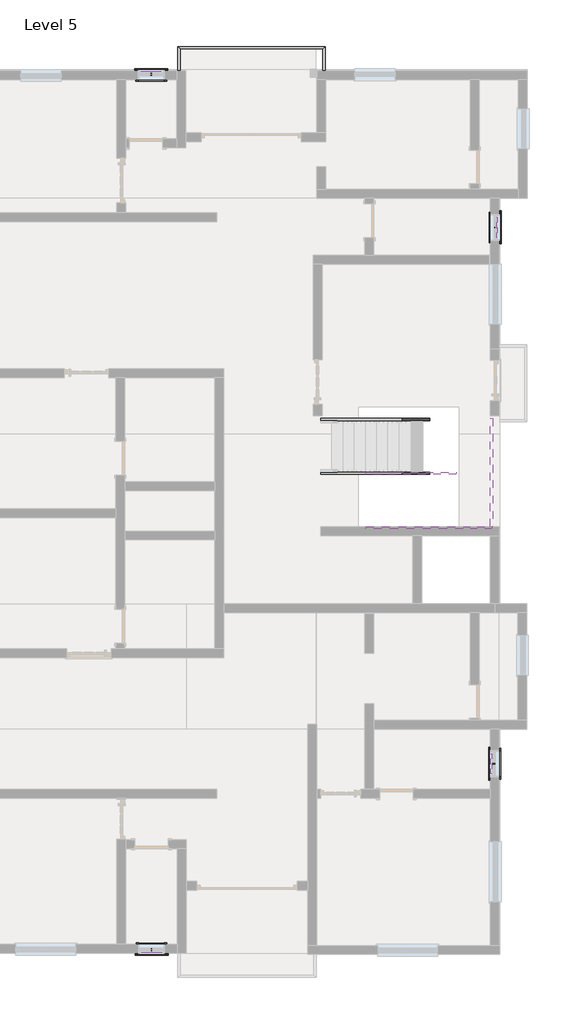
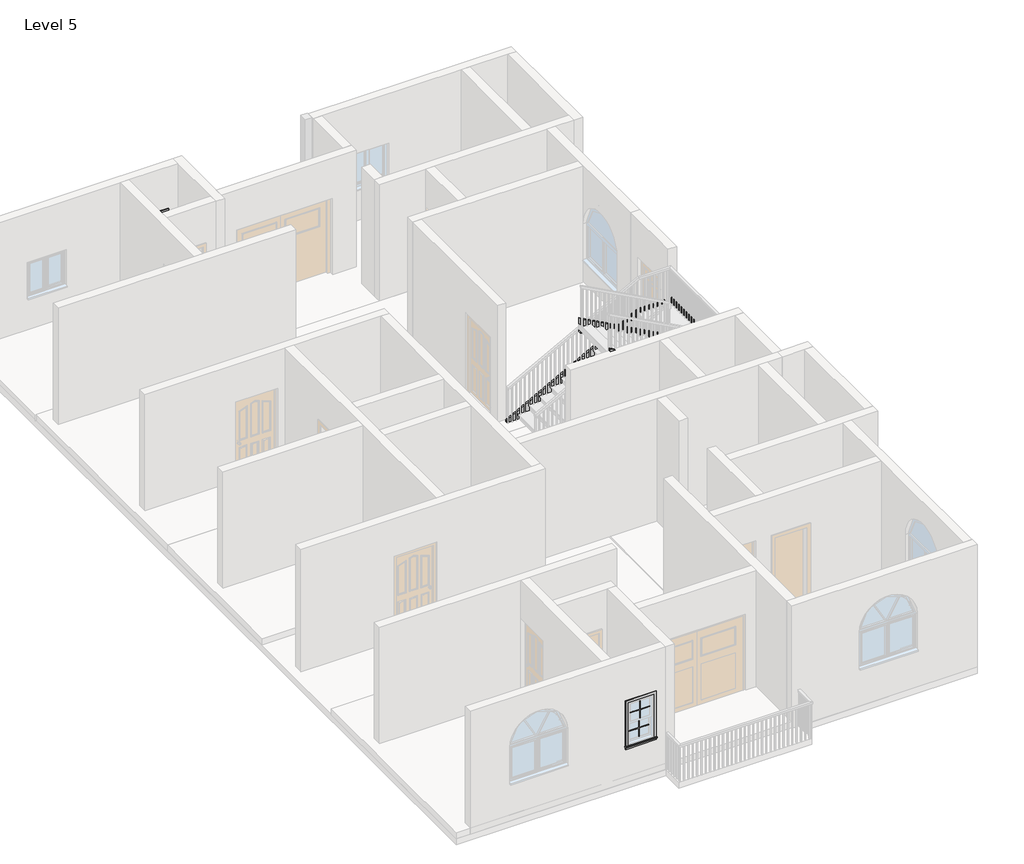
# One storey, part 7 of 7: 16 proxies, 5 members, 1 railing.
"""IFC4 building model written with IfcOpenShell, lengths in millimetres."""

from ifc_helpers import new_model, si_unit, frame, origin, place, context, project, spatial, polyline, outline, extrude, faceted_brep, transform, mapped, element, save
from components import muntin_pattern_2x2_muntin_pattern_2x2_eba6c5fb, trim_window_exterior_flat_with_sill_278e6a94, trim_window_interior_flat_picture_frame_e9fd5f45

model = new_model("IFC4")

# Units and contexts
model_context = context("Model", 3, world=origin())
ifc_project = project(units=[si_unit("LENGTHUNIT", "METRE", prefix="MILLI")], contexts=[model_context])

# Site, building, storey
site = spatial("IfcSite", under=ifc_project)
building = spatial("IfcBuilding", under=site)
storey = spatial("IfcBuildingStorey", under=building, Name="Level 5", Elevation=12192.0)

# Proxies
placement = place(None, origin())
muntin_pattern_2x2_muntin_pattern_2x2_shape = muntin_pattern_2x2_muntin_pattern_2x2_eba6c5fb(model_context)
element("IfcBuildingElementProxy", 1, Name="Muntin Pattern_2x2 : Muntin Pattern_2x2", ObjectType="Muntin Pattern_2x2 : Muntin Pattern_2x2", at=placement, inside=storey, context=model_context, shape_type="MappedRepresentation", body=[
    mapped(muntin_pattern_2x2_muntin_pattern_2x2_shape, transform((5828.2640963, 5846.2962251, 13662.025), x_axis=(0.0, -1.0, 0.0), y_axis=(1.0, 0.0, 0.0), z_axis=(0.0, 0.0, 1.0))),
])
element("IfcBuildingElementProxy", 2, Name="Muntin Pattern_2x2 : Muntin Pattern_2x2", ObjectType="Muntin Pattern_2x2 : Muntin Pattern_2x2", at=placement, inside=storey, context=model_context, shape_type="MappedRepresentation", body=[
    mapped(muntin_pattern_2x2_muntin_pattern_2x2_shape, transform((5783.8140963, 5846.2962251, 13182.6), x_axis=(0.0, -1.0, 0.0), y_axis=(1.0, 0.0, 0.0), z_axis=(0.0, 0.0, 1.0))),
])
element("IfcBuildingElementProxy", 3, Name="Muntin Pattern_2x2 : Muntin Pattern_2x2", ObjectType="Muntin Pattern_2x2 : Muntin Pattern_2x2", at=placement, inside=storey, context=model_context, shape_type="MappedRepresentation", body=[
    mapped(muntin_pattern_2x2_muntin_pattern_2x2_shape, transform((5694.9140963, -6313.9537749, 13662.025), x_axis=(0.0, 1.0, 0.0), y_axis=(-1.0, 0.0, 0.0), z_axis=(0.0, 0.0, 1.0))),
])
element("IfcBuildingElementProxy", 4, Name="Muntin Pattern_2x2 : Muntin Pattern_2x2", ObjectType="Muntin Pattern_2x2 : Muntin Pattern_2x2", at=placement, inside=storey, context=model_context, shape_type="MappedRepresentation", body=[
    mapped(muntin_pattern_2x2_muntin_pattern_2x2_shape, transform((5739.3640963, -6313.9537749, 13182.6), x_axis=(0.0, 1.0, 0.0), y_axis=(-1.0, 0.0, 0.0), z_axis=(0.0, 0.0, 1.0))),
])
element("IfcBuildingElementProxy", 5, Name="Muntin Pattern_2x2 : Muntin Pattern_2x2", ObjectType="Muntin Pattern_2x2 : Muntin Pattern_2x2", at=placement, inside=storey, context=model_context, shape_type="MappedRepresentation", body=[
    mapped(muntin_pattern_2x2_muntin_pattern_2x2_shape, transform((-2029.8609037, 9366.9277313, 13662.025), x_axis=(1.0, 0.0, 0.0), y_axis=(0.0, 1.0, 0.0), z_axis=(0.0, 0.0, 1.0))),
])
element("IfcBuildingElementProxy", 6, Name="Muntin Pattern_2x2 : Muntin Pattern_2x2", ObjectType="Muntin Pattern_2x2 : Muntin Pattern_2x2", at=placement, inside=storey, context=model_context, shape_type="MappedRepresentation", body=[
    mapped(muntin_pattern_2x2_muntin_pattern_2x2_shape, transform((-2029.8609037, 9322.4777313, 13182.6), x_axis=(1.0, 0.0, 0.0), y_axis=(0.0, 1.0, 0.0), z_axis=(0.0, 0.0, 1.0))),
])
element("IfcBuildingElementProxy", 7, Name="Muntin Pattern_2x2 : Muntin Pattern_2x2", ObjectType="Muntin Pattern_2x2 : Muntin Pattern_2x2", at=placement, inside=storey, context=model_context, shape_type="MappedRepresentation", body=[
    mapped(muntin_pattern_2x2_muntin_pattern_2x2_shape, transform((-2023.5109037, -10577.9787749, 13662.025), x_axis=(-1.0, 0.0, 0.0), y_axis=(0.0, -1.0, 0.0), z_axis=(0.0, 0.0, 1.0))),
])
element("IfcBuildingElementProxy", 8, Name="Muntin Pattern_2x2 : Muntin Pattern_2x2", ObjectType="Muntin Pattern_2x2 : Muntin Pattern_2x2", at=placement, inside=storey, context=model_context, shape_type="MappedRepresentation", body=[
    mapped(muntin_pattern_2x2_muntin_pattern_2x2_shape, transform((-2023.5109037, -10533.5287749, 13182.6), x_axis=(-1.0, 0.0, 0.0), y_axis=(0.0, -1.0, 0.0), z_axis=(0.0, 0.0, 1.0))),
])
trim_window_exterior_flat_with_sill_shape = trim_window_exterior_flat_with_sill_278e6a94(model_context)
element("IfcBuildingElementProxy", 9, Name="Trim-Window-Exterior-Flat : with Sill", ObjectType="Trim-Window-Exterior-Flat : with Sill", at=placement, inside=storey, context=model_context, shape_type="MappedRepresentation", body=[
    mapped(trim_window_exterior_flat_with_sill_shape, transform((5863.1890963, 5846.2962251, 14173.2), x_axis=(0.0, 1.0, 0.0), y_axis=(0.0, 0.0, 1.0), z_axis=(1.0, 0.0, 0.0))),
])
element("IfcBuildingElementProxy", 10, Name="Trim-Window-Exterior-Flat : with Sill", ObjectType="Trim-Window-Exterior-Flat : with Sill", at=placement, inside=storey, context=model_context, shape_type="MappedRepresentation", body=[
    mapped(trim_window_exterior_flat_with_sill_shape, transform((5659.9890963, -6313.9537749, 14173.2), x_axis=(0.0, -1.0, 0.0), y_axis=(0.0, 0.0, 1.0), z_axis=(-1.0, 0.0, 0.0))),
])
element("IfcBuildingElementProxy", 11, Name="Trim-Window-Exterior-Flat : with Sill", ObjectType="Trim-Window-Exterior-Flat : with Sill", at=placement, inside=storey, context=model_context, shape_type="MappedRepresentation", body=[
    mapped(trim_window_exterior_flat_with_sill_shape, transform((-2029.8609037, 9401.8527313, 14173.2), x_axis=(-1.0, 0.0, 0.0), y_axis=(0.0, 0.0, 1.0), z_axis=(0.0, 1.0, 0.0))),
])
element("IfcBuildingElementProxy", 12, Name="Trim-Window-Exterior-Flat : with Sill", ObjectType="Trim-Window-Exterior-Flat : with Sill", at=placement, inside=storey, context=model_context, shape_type="MappedRepresentation", body=[
    mapped(trim_window_exterior_flat_with_sill_shape, transform((-2023.5109037, -10612.9037749, 14173.2), x_axis=(1.0, 0.0, 0.0), y_axis=(0.0, 0.0, 1.0), z_axis=(0.0, -1.0, 0.0))),
])
trim_window_interior_flat_picture_frame_shape = trim_window_interior_flat_picture_frame_e9fd5f45(model_context)
element("IfcBuildingElementProxy", 13, Name="Trim-Window-Interior-Flat : Picture Frame", ObjectType="Trim-Window-Interior-Flat : Picture Frame", at=placement, inside=storey, context=model_context, shape_type="MappedRepresentation", body=[
    mapped(trim_window_interior_flat_picture_frame_shape, transform((5659.9890963, 5846.2962251, 14173.2), x_axis=(0.0, -1.0, 0.0), y_axis=(0.0, 0.0, 1.0), z_axis=(-1.0, 0.0, 0.0))),
])
element("IfcBuildingElementProxy", 14, Name="Trim-Window-Interior-Flat : Picture Frame", ObjectType="Trim-Window-Interior-Flat : Picture Frame", at=placement, inside=storey, context=model_context, shape_type="MappedRepresentation", body=[
    mapped(trim_window_interior_flat_picture_frame_shape, transform((5863.1890963, -6313.9537749, 14173.2), x_axis=(0.0, 1.0, 0.0), y_axis=(0.0, 0.0, 1.0), z_axis=(1.0, 0.0, 0.0))),
])
element("IfcBuildingElementProxy", 15, Name="Trim-Window-Interior-Flat : Picture Frame", ObjectType="Trim-Window-Interior-Flat : Picture Frame", at=placement, inside=storey, context=model_context, shape_type="MappedRepresentation", body=[
    mapped(trim_window_interior_flat_picture_frame_shape, transform((-2029.8609037, 9198.6527313, 14173.2), x_axis=(1.0, 0.0, 0.0), y_axis=(0.0, 0.0, 1.0), z_axis=(0.0, -1.0, 0.0))),
])
element("IfcBuildingElementProxy", 16, Name="Trim-Window-Interior-Flat : Picture Frame", ObjectType="Trim-Window-Interior-Flat : Picture Frame", at=placement, inside=storey, context=model_context, shape_type="MappedRepresentation", body=[
    mapped(trim_window_interior_flat_picture_frame_shape, transform((-2023.5109037, -10409.7037749, 14173.2), x_axis=(-1.0, 0.0, 0.0), y_axis=(0.0, 0.0, 1.0), z_axis=(0.0, 1.0, 0.0))),
])

# Members
element("IfcMember", 17, ObjectType="Stringer - 2\" Width", at=placement, inside=storey, context=model_context, shape_type="SweptSolid", body=[
    extrude(outline(polyline([(12399.4423129, 1811.8890963), (12192.0, 1811.8890963), (12192.0, 2068.9379367), (14069.2909091, 5536.6829612), (14069.2909091, 4896.4452154), (12399.4423129, 1811.8890963)])), frame((0.0, 1464.7962251, 0.0), z_axis=(0.0, 1.0, 0.0), x_axis=(0.0, 0.0, 1.0)), (0.0, 0.0, 1.0), 50.8),
])
element("IfcMember", 18, ObjectType="Stringer - 2\" Width", at=placement, inside=storey, context=model_context, shape_type="SweptSolid", body=[
    extrude(outline(polyline([(5659.9890963, 1515.5962251), (5710.7890963, 1515.5962251), (5710.7890963, -935.5037749), (5659.9890963, -935.5037749), (5659.9890963, 1515.5962251)])), frame((0.0, 0.0, 13764.4909091), z_axis=(0.0, 0.0, 1.0), x_axis=(1.0, 0.0, 0.0)), (0.0, 0.0, 1.0), 304.8),
])
element("IfcMember", 19, ObjectType="Stringer - 2\" Width", at=placement, inside=storey, context=model_context, shape_type="SweptSolid", body=[
    extrude(outline(polyline([(13764.4909091, 5687.6636359), (15306.0362324, 2827.8890963), (14959.7736638, 2827.8890963), (13764.4909091, 5045.2998579), (13764.4909091, 5687.6636359)])), frame((0.0, -986.3037749, 0.0), z_axis=(0.0, 1.0, 0.0), x_axis=(0.0, 0.0, 1.0)), (0.0, 0.0, 1.0), 50.8),
])
element("IfcMember", 20, ObjectType="Stringer - 2\" Width", at=placement, inside=storey, context=model_context, shape_type="SweptSolid", body=[
    extrude(outline(polyline([(12399.4423129, 1811.8890963), (12192.0, 1811.8890963), (12192.0, 2068.9379367), (13686.8485088, 4830.2326586), (14033.4462232, 4830.2326586), (12399.4423129, 1811.8890963)])), frame((0.0, 245.5962251, 0.0), z_axis=(0.0, 1.0, 0.0), x_axis=(0.0, 0.0, 1.0)), (0.0, 0.0, 1.0), 50.8),
])
element("IfcMember", 21, ObjectType="Stringer - 2\" Width", at=placement, inside=storey, context=model_context, shape_type="SweptSolid", body=[
    extrude(outline(polyline([(13853.0382157, 4881.0326586), (14199.3007843, 4881.0326586), (15306.0362324, 2827.8890963), (14959.7736638, 2827.8890963), (13853.0382157, 4881.0326586)])), frame((0.0, 245.5962251, 0.0), z_axis=(0.0, 1.0, 0.0), x_axis=(0.0, 0.0, 1.0)), (0.0, 0.0, 1.0), 50.8),
])

# Railing
element("IfcRailing", 22, ObjectType="Handrail - Rectangular", at=placement, inside=storey, context=model_context, shape_type="SolidModel", body=[
    faceted_brep([(-1426.6109037, 9402.2962251, 13106.4), (-1426.6109037, 9402.2962251, 13055.6), (-1375.8109037, 9402.2962251, 13055.6), (-1375.8109037, 9402.2962251, 13106.4), (-1426.6109037, 9948.3962251, 13106.4), (-1426.6109037, 9948.3962251, 13055.6), (-1375.8109037, 9897.5962251, 13055.6), (-1375.8109037, 9897.5962251, 13106.4), (1913.4890963, 9948.3962251, 13106.4), (1913.4890963, 9948.3962251, 13055.6), (1862.6890963, 9897.5962251, 13055.6), (1862.6890963, 9897.5962251, 13106.4), (1913.4890963, 9402.2962251, 13106.4), (1862.6890963, 9402.2962251, 13106.4), (1862.6890963, 9402.2962251, 13055.6), (1913.4890963, 9402.2962251, 13055.6)], [[[0, 1, 2, 3]], [[1, 0, 4, 5]], [[2, 1, 5, 6]], [[3, 2, 6, 7]], [[0, 3, 7, 4]], [[5, 4, 8, 9]], [[6, 5, 9, 10]], [[7, 6, 10, 11]], [[4, 7, 11, 8]], [[12, 13, 14, 15]], [[9, 8, 12, 15]], [[10, 9, 15, 14]], [[11, 10, 14, 13]], [[8, 11, 13, 12]]]),
    extrude(outline(polyline([(1878.5640963, 9424.5212251), (1897.6140963, 9424.5212251), (1897.6140963, 9405.4712251), (1878.5640963, 9405.4712251), (1878.5640963, 9424.5212251)])), frame((0.0, 0.0, 12192.0), z_axis=(0.0, 0.0, 1.0), x_axis=(1.0, 0.0, 0.0)), (0.0, 0.0, 1.0), 863.6),
    extrude(outline(polyline([(1878.5640963, 9526.1212251), (1897.6140963, 9526.1212251), (1897.6140963, 9507.0712251), (1878.5640963, 9507.0712251), (1878.5640963, 9526.1212251)])), frame((0.0, 0.0, 12192.0), z_axis=(0.0, 0.0, 1.0), x_axis=(1.0, 0.0, 0.0)), (0.0, 0.0, 1.0), 863.6),
    extrude(outline(polyline([(1878.5640963, 9627.7212251), (1897.6140963, 9627.7212251), (1897.6140963, 9608.6712251), (1878.5640963, 9608.6712251), (1878.5640963, 9627.7212251)])), frame((0.0, 0.0, 12192.0), z_axis=(0.0, 0.0, 1.0), x_axis=(1.0, 0.0, 0.0)), (0.0, 0.0, 1.0), 863.6),
    extrude(outline(polyline([(1878.5640963, 9729.3212251), (1897.6140963, 9729.3212251), (1897.6140963, 9710.2712251), (1878.5640963, 9710.2712251), (1878.5640963, 9729.3212251)])), frame((0.0, 0.0, 12192.0), z_axis=(0.0, 0.0, 1.0), x_axis=(1.0, 0.0, 0.0)), (0.0, 0.0, 1.0), 863.6),
    extrude(outline(polyline([(1878.5640963, 9830.9212251), (1897.6140963, 9830.9212251), (1897.6140963, 9811.8712251), (1878.5640963, 9811.8712251), (1878.5640963, 9830.9212251)])), frame((0.0, 0.0, 12192.0), z_axis=(0.0, 0.0, 1.0), x_axis=(1.0, 0.0, 0.0)), (0.0, 0.0, 1.0), 863.6),
    extrude(outline(polyline([(1840.4640963, 9913.4712251), (1840.4640963, 9932.5212251), (1859.5140963, 9932.5212251), (1859.5140963, 9913.4712251), (1840.4640963, 9913.4712251)])), frame((0.0, 0.0, 12192.0), z_axis=(0.0, 0.0, 1.0), x_axis=(1.0, 0.0, 0.0)), (0.0, 0.0, 1.0), 863.6),
    extrude(outline(polyline([(1738.8640963, 9913.4712251), (1738.8640963, 9932.5212251), (1757.9140963, 9932.5212251), (1757.9140963, 9913.4712251), (1738.8640963, 9913.4712251)])), frame((0.0, 0.0, 12192.0), z_axis=(0.0, 0.0, 1.0), x_axis=(1.0, 0.0, 0.0)), (0.0, 0.0, 1.0), 863.6),
    extrude(outline(polyline([(1637.2640963, 9913.4712251), (1637.2640963, 9932.5212251), (1656.3140963, 9932.5212251), (1656.3140963, 9913.4712251), (1637.2640963, 9913.4712251)])), frame((0.0, 0.0, 12192.0), z_axis=(0.0, 0.0, 1.0), x_axis=(1.0, 0.0, 0.0)), (0.0, 0.0, 1.0), 863.6),
    extrude(outline(polyline([(1535.6640963, 9913.4712251), (1535.6640963, 9932.5212251), (1554.7140963, 9932.5212251), (1554.7140963, 9913.4712251), (1535.6640963, 9913.4712251)])), frame((0.0, 0.0, 12192.0), z_axis=(0.0, 0.0, 1.0), x_axis=(1.0, 0.0, 0.0)), (0.0, 0.0, 1.0), 863.6),
    extrude(outline(polyline([(1434.0640963, 9913.4712251), (1434.0640963, 9932.5212251), (1453.1140963, 9932.5212251), (1453.1140963, 9913.4712251), (1434.0640963, 9913.4712251)])), frame((0.0, 0.0, 12192.0), z_axis=(0.0, 0.0, 1.0), x_axis=(1.0, 0.0, 0.0)), (0.0, 0.0, 1.0), 863.6),
    extrude(outline(polyline([(1332.4640963, 9913.4712251), (1332.4640963, 9932.5212251), (1351.5140963, 9932.5212251), (1351.5140963, 9913.4712251), (1332.4640963, 9913.4712251)])), frame((0.0, 0.0, 12192.0), z_axis=(0.0, 0.0, 1.0), x_axis=(1.0, 0.0, 0.0)), (0.0, 0.0, 1.0), 863.6),
    extrude(outline(polyline([(1230.8640963, 9913.4712251), (1230.8640963, 9932.5212251), (1249.9140963, 9932.5212251), (1249.9140963, 9913.4712251), (1230.8640963, 9913.4712251)])), frame((0.0, 0.0, 12192.0), z_axis=(0.0, 0.0, 1.0), x_axis=(1.0, 0.0, 0.0)), (0.0, 0.0, 1.0), 863.6),
    extrude(outline(polyline([(1129.2640963, 9913.4712251), (1129.2640963, 9932.5212251), (1148.3140963, 9932.5212251), (1148.3140963, 9913.4712251), (1129.2640963, 9913.4712251)])), frame((0.0, 0.0, 12192.0), z_axis=(0.0, 0.0, 1.0), x_axis=(1.0, 0.0, 0.0)), (0.0, 0.0, 1.0), 863.6),
    extrude(outline(polyline([(1027.6640963, 9913.4712251), (1027.6640963, 9932.5212251), (1046.7140963, 9932.5212251), (1046.7140963, 9913.4712251), (1027.6640963, 9913.4712251)])), frame((0.0, 0.0, 12192.0), z_axis=(0.0, 0.0, 1.0), x_axis=(1.0, 0.0, 0.0)), (0.0, 0.0, 1.0), 863.6),
    extrude(outline(polyline([(926.0640963, 9913.4712251), (926.0640963, 9932.5212251), (945.1140963, 9932.5212251), (945.1140963, 9913.4712251), (926.0640963, 9913.4712251)])), frame((0.0, 0.0, 12192.0), z_axis=(0.0, 0.0, 1.0), x_axis=(1.0, 0.0, 0.0)), (0.0, 0.0, 1.0), 863.6),
    extrude(outline(polyline([(824.4640963, 9913.4712251), (824.4640963, 9932.5212251), (843.5140963, 9932.5212251), (843.5140963, 9913.4712251), (824.4640963, 9913.4712251)])), frame((0.0, 0.0, 12192.0), z_axis=(0.0, 0.0, 1.0), x_axis=(1.0, 0.0, 0.0)), (0.0, 0.0, 1.0), 863.6),
    extrude(outline(polyline([(722.8640963, 9913.4712251), (722.8640963, 9932.5212251), (741.9140963, 9932.5212251), (741.9140963, 9913.4712251), (722.8640963, 9913.4712251)])), frame((0.0, 0.0, 12192.0), z_axis=(0.0, 0.0, 1.0), x_axis=(1.0, 0.0, 0.0)), (0.0, 0.0, 1.0), 863.6),
    extrude(outline(polyline([(621.2640963, 9913.4712251), (621.2640963, 9932.5212251), (640.3140963, 9932.5212251), (640.3140963, 9913.4712251), (621.2640963, 9913.4712251)])), frame((0.0, 0.0, 12192.0), z_axis=(0.0, 0.0, 1.0), x_axis=(1.0, 0.0, 0.0)), (0.0, 0.0, 1.0), 863.6),
    extrude(outline(polyline([(519.6640963, 9913.4712251), (519.6640963, 9932.5212251), (538.7140963, 9932.5212251), (538.7140963, 9913.4712251), (519.6640963, 9913.4712251)])), frame((0.0, 0.0, 12192.0), z_axis=(0.0, 0.0, 1.0), x_axis=(1.0, 0.0, 0.0)), (0.0, 0.0, 1.0), 863.6),
    extrude(outline(polyline([(418.0640963, 9913.4712251), (418.0640963, 9932.5212251), (437.1140963, 9932.5212251), (437.1140963, 9913.4712251), (418.0640963, 9913.4712251)])), frame((0.0, 0.0, 12192.0), z_axis=(0.0, 0.0, 1.0), x_axis=(1.0, 0.0, 0.0)), (0.0, 0.0, 1.0), 863.6),
    extrude(outline(polyline([(316.4640963, 9913.4712251), (316.4640963, 9932.5212251), (335.5140963, 9932.5212251), (335.5140963, 9913.4712251), (316.4640963, 9913.4712251)])), frame((0.0, 0.0, 12192.0), z_axis=(0.0, 0.0, 1.0), x_axis=(1.0, 0.0, 0.0)), (0.0, 0.0, 1.0), 863.6),
    extrude(outline(polyline([(214.8640963, 9913.4712251), (214.8640963, 9932.5212251), (233.9140963, 9932.5212251), (233.9140963, 9913.4712251), (214.8640963, 9913.4712251)])), frame((0.0, 0.0, 12192.0), z_axis=(0.0, 0.0, 1.0), x_axis=(1.0, 0.0, 0.0)), (0.0, 0.0, 1.0), 863.6),
    extrude(outline(polyline([(113.2640963, 9913.4712251), (113.2640963, 9932.5212251), (132.3140963, 9932.5212251), (132.3140963, 9913.4712251), (113.2640963, 9913.4712251)])), frame((0.0, 0.0, 12192.0), z_axis=(0.0, 0.0, 1.0), x_axis=(1.0, 0.0, 0.0)), (0.0, 0.0, 1.0), 863.6),
    extrude(outline(polyline([(11.6640963, 9913.4712251), (11.6640963, 9932.5212251), (30.7140963, 9932.5212251), (30.7140963, 9913.4712251), (11.6640963, 9913.4712251)])), frame((0.0, 0.0, 12192.0), z_axis=(0.0, 0.0, 1.0), x_axis=(1.0, 0.0, 0.0)), (0.0, 0.0, 1.0), 863.6),
    extrude(outline(polyline([(-89.9359037, 9913.4712251), (-89.9359037, 9932.5212251), (-70.8859037, 9932.5212251), (-70.8859037, 9913.4712251), (-89.9359037, 9913.4712251)])), frame((0.0, 0.0, 12192.0), z_axis=(0.0, 0.0, 1.0), x_axis=(1.0, 0.0, 0.0)), (0.0, 0.0, 1.0), 863.6),
    extrude(outline(polyline([(-191.5359037, 9913.4712251), (-191.5359037, 9932.5212251), (-172.4859037, 9932.5212251), (-172.4859037, 9913.4712251), (-191.5359037, 9913.4712251)])), frame((0.0, 0.0, 12192.0), z_axis=(0.0, 0.0, 1.0), x_axis=(1.0, 0.0, 0.0)), (0.0, 0.0, 1.0), 863.6),
    extrude(outline(polyline([(-293.1359037, 9913.4712251), (-293.1359037, 9932.5212251), (-274.0859037, 9932.5212251), (-274.0859037, 9913.4712251), (-293.1359037, 9913.4712251)])), frame((0.0, 0.0, 12192.0), z_axis=(0.0, 0.0, 1.0), x_axis=(1.0, 0.0, 0.0)), (0.0, 0.0, 1.0), 863.6),
    extrude(outline(polyline([(-394.7359037, 9913.4712251), (-394.7359037, 9932.5212251), (-375.6859037, 9932.5212251), (-375.6859037, 9913.4712251), (-394.7359037, 9913.4712251)])), frame((0.0, 0.0, 12192.0), z_axis=(0.0, 0.0, 1.0), x_axis=(1.0, 0.0, 0.0)), (0.0, 0.0, 1.0), 863.6),
    extrude(outline(polyline([(-496.3359037, 9913.4712251), (-496.3359037, 9932.5212251), (-477.2859037, 9932.5212251), (-477.2859037, 9913.4712251), (-496.3359037, 9913.4712251)])), frame((0.0, 0.0, 12192.0), z_axis=(0.0, 0.0, 1.0), x_axis=(1.0, 0.0, 0.0)), (0.0, 0.0, 1.0), 863.6),
    extrude(outline(polyline([(-597.9359037, 9913.4712251), (-597.9359037, 9932.5212251), (-578.8859037, 9932.5212251), (-578.8859037, 9913.4712251), (-597.9359037, 9913.4712251)])), frame((0.0, 0.0, 12192.0), z_axis=(0.0, 0.0, 1.0), x_axis=(1.0, 0.0, 0.0)), (0.0, 0.0, 1.0), 863.6),
    extrude(outline(polyline([(-699.5359037, 9913.4712251), (-699.5359037, 9932.5212251), (-680.4859037, 9932.5212251), (-680.4859037, 9913.4712251), (-699.5359037, 9913.4712251)])), frame((0.0, 0.0, 12192.0), z_axis=(0.0, 0.0, 1.0), x_axis=(1.0, 0.0, 0.0)), (0.0, 0.0, 1.0), 863.6),
    extrude(outline(polyline([(-801.1359037, 9913.4712251), (-801.1359037, 9932.5212251), (-782.0859037, 9932.5212251), (-782.0859037, 9913.4712251), (-801.1359037, 9913.4712251)])), frame((0.0, 0.0, 12192.0), z_axis=(0.0, 0.0, 1.0), x_axis=(1.0, 0.0, 0.0)), (0.0, 0.0, 1.0), 863.6),
    extrude(outline(polyline([(-902.7359037, 9913.4712251), (-902.7359037, 9932.5212251), (-883.6859037, 9932.5212251), (-883.6859037, 9913.4712251), (-902.7359037, 9913.4712251)])), frame((0.0, 0.0, 12192.0), z_axis=(0.0, 0.0, 1.0), x_axis=(1.0, 0.0, 0.0)), (0.0, 0.0, 1.0), 863.6),
    extrude(outline(polyline([(-1004.3359037, 9913.4712251), (-1004.3359037, 9932.5212251), (-985.2859037, 9932.5212251), (-985.2859037, 9913.4712251), (-1004.3359037, 9913.4712251)])), frame((0.0, 0.0, 12192.0), z_axis=(0.0, 0.0, 1.0), x_axis=(1.0, 0.0, 0.0)), (0.0, 0.0, 1.0), 863.6),
    extrude(outline(polyline([(-1105.9359037, 9913.4712251), (-1105.9359037, 9932.5212251), (-1086.8859037, 9932.5212251), (-1086.8859037, 9913.4712251), (-1105.9359037, 9913.4712251)])), frame((0.0, 0.0, 12192.0), z_axis=(0.0, 0.0, 1.0), x_axis=(1.0, 0.0, 0.0)), (0.0, 0.0, 1.0), 863.6),
    extrude(outline(polyline([(-1207.5359037, 9913.4712251), (-1207.5359037, 9932.5212251), (-1188.4859037, 9932.5212251), (-1188.4859037, 9913.4712251), (-1207.5359037, 9913.4712251)])), frame((0.0, 0.0, 12192.0), z_axis=(0.0, 0.0, 1.0), x_axis=(1.0, 0.0, 0.0)), (0.0, 0.0, 1.0), 863.6),
    extrude(outline(polyline([(-1309.1359037, 9913.4712251), (-1309.1359037, 9932.5212251), (-1290.0859037, 9932.5212251), (-1290.0859037, 9913.4712251), (-1309.1359037, 9913.4712251)])), frame((0.0, 0.0, 12192.0), z_axis=(0.0, 0.0, 1.0), x_axis=(1.0, 0.0, 0.0)), (0.0, 0.0, 1.0), 863.6),
    extrude(outline(polyline([(-1391.6859037, 9900.7712251), (-1410.7359037, 9900.7712251), (-1410.7359037, 9919.8212251), (-1391.6859037, 9919.8212251), (-1391.6859037, 9900.7712251)])), frame((0.0, 0.0, 12192.0), z_axis=(0.0, 0.0, 1.0), x_axis=(1.0, 0.0, 0.0)), (0.0, 0.0, 1.0), 863.6),
    extrude(outline(polyline([(-1391.6859037, 9799.1712251), (-1410.7359037, 9799.1712251), (-1410.7359037, 9818.2212251), (-1391.6859037, 9818.2212251), (-1391.6859037, 9799.1712251)])), frame((0.0, 0.0, 12192.0), z_axis=(0.0, 0.0, 1.0), x_axis=(1.0, 0.0, 0.0)), (0.0, 0.0, 1.0), 863.6),
    extrude(outline(polyline([(-1391.6859037, 9697.5712251), (-1410.7359037, 9697.5712251), (-1410.7359037, 9716.6212251), (-1391.6859037, 9716.6212251), (-1391.6859037, 9697.5712251)])), frame((0.0, 0.0, 12192.0), z_axis=(0.0, 0.0, 1.0), x_axis=(1.0, 0.0, 0.0)), (0.0, 0.0, 1.0), 863.6),
    extrude(outline(polyline([(-1391.6859037, 9595.9712251), (-1410.7359037, 9595.9712251), (-1410.7359037, 9615.0212251), (-1391.6859037, 9615.0212251), (-1391.6859037, 9595.9712251)])), frame((0.0, 0.0, 12192.0), z_axis=(0.0, 0.0, 1.0), x_axis=(1.0, 0.0, 0.0)), (0.0, 0.0, 1.0), 863.6),
    extrude(outline(polyline([(-1391.6859037, 9494.3712251), (-1410.7359037, 9494.3712251), (-1410.7359037, 9513.4212251), (-1391.6859037, 9513.4212251), (-1391.6859037, 9494.3712251)])), frame((0.0, 0.0, 12192.0), z_axis=(0.0, 0.0, 1.0), x_axis=(1.0, 0.0, 0.0)), (0.0, 0.0, 1.0), 863.6),
    extrude(outline(polyline([(1878.5640963, 9913.4712251), (1878.5640963, 9932.5212251), (1897.6140963, 9932.5212251), (1897.6140963, 9913.4712251), (1878.5640963, 9913.4712251)])), frame((0.0, 0.0, 12192.0), z_axis=(0.0, 0.0, 1.0), x_axis=(1.0, 0.0, 0.0)), (0.0, 0.0, 1.0), 863.6),
    extrude(outline(polyline([(-1391.6859037, 9913.4712251), (-1410.7359037, 9913.4712251), (-1410.7359037, 9932.5212251), (-1391.6859037, 9932.5212251), (-1391.6859037, 9913.4712251)])), frame((0.0, 0.0, 12192.0), z_axis=(0.0, 0.0, 1.0), x_axis=(1.0, 0.0, 0.0)), (0.0, 0.0, 1.0), 863.6),
    extrude(outline(polyline([(1878.5640963, 9421.3462251), (1897.6140963, 9421.3462251), (1897.6140963, 9402.2962251), (1878.5640963, 9402.2962251), (1878.5640963, 9421.3462251)])), frame((0.0, 0.0, 12192.0), z_axis=(0.0, 0.0, 1.0), x_axis=(1.0, 0.0, 0.0)), (0.0, 0.0, 1.0), 863.6),
    extrude(outline(polyline([(-1391.6859037, 9402.2962251), (-1410.7359037, 9402.2962251), (-1410.7359037, 9421.3462251), (-1391.6859037, 9421.3462251), (-1391.6859037, 9402.2962251)])), frame((0.0, 0.0, 12192.0), z_axis=(0.0, 0.0, 1.0), x_axis=(1.0, 0.0, 0.0)), (0.0, 0.0, 1.0), 863.6),
])

save(model, "model.ifc")

# Revit data of these elements
# Type "Muntin Pattern_2x2 : Muntin Pattern_2x2"
#   Width [instance default] = 4' - 0"
#   Thickness = 0' - 0 1/2"
#   Height [instance default] = 4' - 0"
#   Distance = 0' - 0 3/4"
#   Interior Material [instance default] = none
#   Exterior Material [instance default] = none
#   Default Elevation = 0
# Type "Trim-Window-Exterior-Flat : with Sill"
#   Trim Width = 0' - 2 1/4"
#   Trim Thickness_Picture Frame = 0' - 1 1/4"
#   Trim Thickness_with Sill = 0' - 0 3/4"
#   Sill Thickness = 0' - 1 1/4"
#   Opening Width [instance default] = 2' - 0"
#   Opening Height [instance default] = 3' - 0"
#   Default Elevation = 4' - 0"
#   Sill = yes
#   Picture Frame = no
#   Trim Material [instance default] = none
# Type "Trim-Window-Interior-Flat : Picture Frame"
#   Trim Thickness_Picture Frame = 0' - 1 1/4"
#   Trim Width = 0' - 2 1/4"
#   Trim Thickness_with Sill = 0' - 0 3/4"
#   Sill Thickness = 0' - 1 1/4"
#   Opening Width [instance default] = 2' - 0"
#   Opening Height [instance default] = 3' - 0"
#   Default Elevation = 4' - 0"
#   Sill = no
#   Picture Frame = yes
#   Trim Material [instance default] = none
# Type "Handrail - Rectangular"
#   Assembly Code = "C2010400"
#   built-in parameter 1008612 = 0.0416667 (stored number, unit not read)
#   built-in parameter 1008611 = 0.0416667 (stored number, unit not read)
#   built-in parameter 1008609 = 0.333333 (stored number, unit not read)
#   built-in parameter 1008604 = 0.166667 (stored number, unit not read)
#   built-in parameter 1008603 = 0.166667 (stored number, unit not read)
#   Railing Height = 3' - 0"
#   built-in parameter 1008630 = 2
#   built-in parameter 1008610 = 2
#   built-in parameter 1008618 = Baluster - Square : 3/4"
# Elements 1, 2, 3, 4, 5, 6, 7, 8 (IfcBuildingElementProxy, "Muntin Pattern_2x2 : Muntin Pattern_2x2")
#   Width = 1' - 6"
#   Height = 1' - 5 1/8"
#   Interior Material = Wood - Stained
#   Exterior Material = Clad - White
#   Phase Created = New Construction
#   Materials on its faces: "Clad - White", "Wood - Stained"
# Elements 9, 10, 11, 12 (IfcBuildingElementProxy, "Trim-Window-Exterior-Flat : with Sill")
#   Opening Width = 2' - 0"
#   Opening Height = 3' - 6"
#   Trim Material = Clad - White
#   Phase Created = New Construction
#   Materials on its faces: "Clad - White"
# Elements 13, 14, 15, 16 (IfcBuildingElementProxy, "Trim-Window-Interior-Flat : Picture Frame")
#   Opening Width = 2' - 0"
#   Opening Height = 3' - 6"
#   Trim Material = Wood - Stained
#   Phase Created = New Construction
#   Materials on its faces: "Wood - Stained"
# Elements 17, 19, 20, 21 (IfcMember, "Stringer - 2\" Width")
#   Phase Created = New Construction
# Element 18 (IfcMember, "Stringer - 2\" Width")
#   Phase Created = New Construction
#   Materials on its faces: "Door - Frame/Mullion"
# Element 22 (IfcRailing, "Handrail - Rectangular")
#   Phase Created = New Construction
# Materials
#   "Clad - White": class "Wood", colour RGB 242 242 238, transparency 0, Cost = 0
#   "Wood - Stained": class "Wood", colour RGB 224 178 126, transparency 0, Cost = 0
#   "Door - Frame/Mullion": class "Wood", colour RGB 212 179 113, transparency 0
